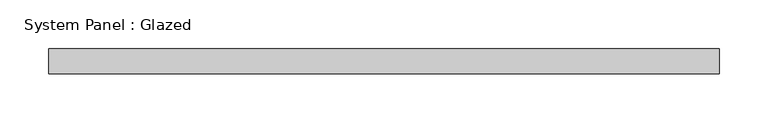
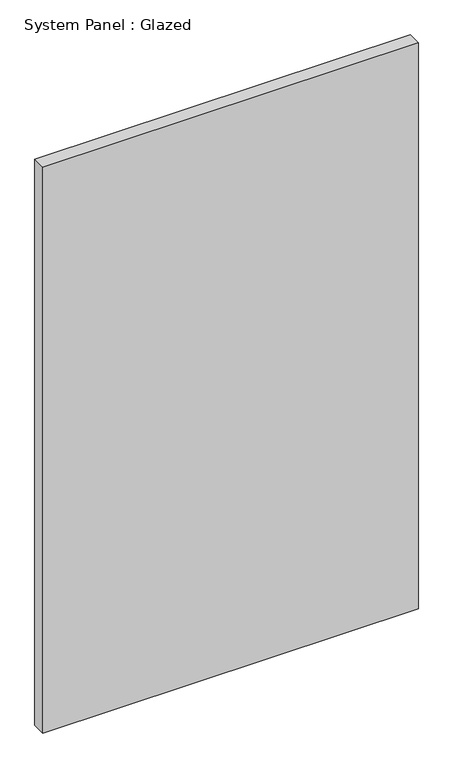
"""IFC4 building model written with IfcOpenShell, lengths in millimetres: plate geometry, System Panel : Glazed."""

from ifc_helpers import new_model, si_unit, origin, origin_with_axes, place, context, project, spatial, polyline, outline, extrude, source, transform, mapped, element, save


def system_panel_glazed_927b5fc9(model_context):
    return source(origin(), model_context, "Body", "SweptSolid", [
        extrude(outline(polyline([(342.9, 19.05), (-342.9, 19.05), (-342.9, 44.45), (342.9, 44.45), (342.9, 19.05)])), origin_with_axes(), (0.0, 0.0, 1.0), 1092.2),
    ])


if __name__ == "__main__":
    model = new_model("IFC4")
    model_context = context("Model", 3, world=origin())
    ifc_project = project(units=[si_unit("LENGTHUNIT", "METRE", prefix="MILLI")], contexts=[model_context])
    site = spatial("IfcSite", under=ifc_project)
    building = spatial("IfcBuilding", under=site)
    placement = place(None, origin())
    system_panel_glazed_shape = system_panel_glazed_927b5fc9(model_context)
    element("IfcPlate", 1, ObjectType="System Panel : Glazed", at=placement, inside=building, context=model_context, shape_type="MappedRepresentation", body=[
        mapped(system_panel_glazed_shape, transform((0.0, 0.0, 0.0), x_axis=(1.0, 0.0, 0.0), y_axis=(0.0, 1.0, 0.0), z_axis=(0.0, 0.0, 1.0))),
    ])
    save(model, "model.ifc")

# Revit data of these elements
# Type "System Panel : Glazed"
#   Construction Type Id = "GSP4R"
#   Analytic Construction = "1/8 in Pilkington single glazing"
#   Visual Light Transmittance = 0.9
#   Solar Heat Gain Coefficient = 0.86
#   Heat Transfer Coefficient (U) = 1.18115 BTU/(h·ft²·°F)
#   Define Thermal Properties by = 1
# Element 1 (IfcPlate, "System Panel : Glazed")
#   Materials on its faces: "Glass"
# Materials
#   "Glass": class "Glass", colour RGB 0 128 192, transparency 0.75, Description = "Soda Lime Glass", Cost = 0
